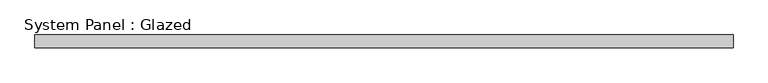
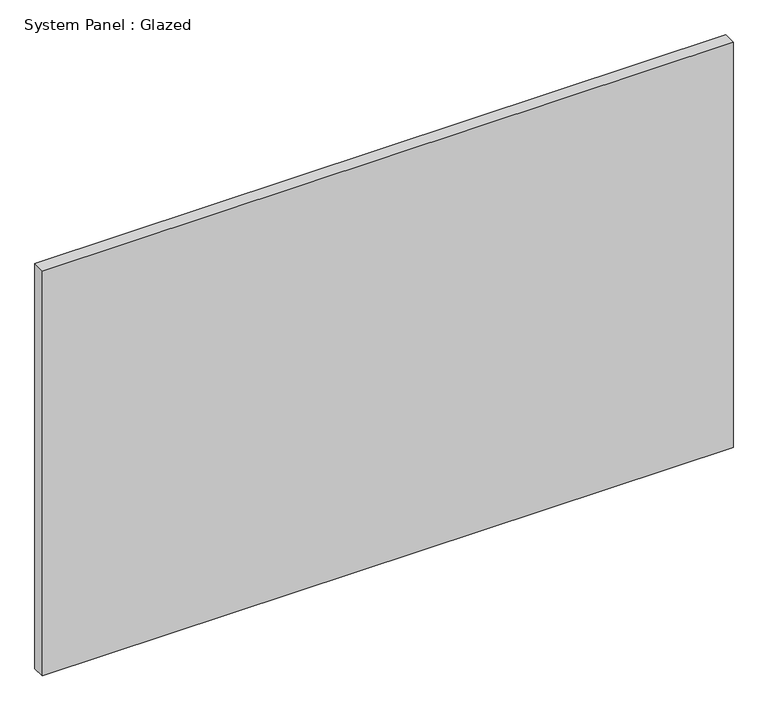
"""IFC4 building model written with IfcOpenShell, lengths in millimetres: plate geometry, System Panel : Glazed."""

from ifc_helpers import new_model, si_unit, origin, origin_with_axes, place, context, project, spatial, polyline, outline, extrude, source, transform, mapped, element, save


def system_panel_glazed_cad8d6ff(model_context):
    return source(origin(), model_context, "Body", "SweptSolid", [
        extrude(outline(polyline([(685.8000001, -44.45), (-685.8000001, -44.45), (-685.8000001, -19.05), (685.8000001, -19.05), (685.8000001, -44.45)])), origin_with_axes(), (0.0, 0.0, 1.0), 850.9),
    ])


if __name__ == "__main__":
    model = new_model("IFC4")
    model_context = context("Model", 3, world=origin())
    ifc_project = project(units=[si_unit("LENGTHUNIT", "METRE", prefix="MILLI")], contexts=[model_context])
    site = spatial("IfcSite", under=ifc_project)
    building = spatial("IfcBuilding", under=site)
    placement = place(None, origin())
    system_panel_glazed_shape = system_panel_glazed_cad8d6ff(model_context)
    element("IfcPlate", 1, ObjectType="System Panel : Glazed", at=placement, inside=building, context=model_context, shape_type="MappedRepresentation", body=[
        mapped(system_panel_glazed_shape, transform((0.0, 0.0, 0.0), x_axis=(1.0, 0.0, 0.0), y_axis=(0.0, 1.0, 0.0), z_axis=(0.0, 0.0, 1.0))),
    ])
    save(model, "model.ifc")

# Revit data of these elements
# Type "System Panel : Glazed"
#   Construction Type Id = "GSP4R"
#   Analytic Construction = "1/8 in Pilkington single glazing"
#   Visual Light Transmittance = 0.9
#   Solar Heat Gain Coefficient = 0.86
#   Heat Transfer Coefficient (U) = 1.18115 BTU/(h·ft²·°F)
#   Define Thermal Properties by = 1
# Element 1 (IfcPlate, "System Panel : Glazed")
#   Materials on its faces: "Glass"
# Materials
#   "Glass": class "Glass", colour RGB 0 128 192, transparency 0.75, Description = "Soda Lime Glass", Cost = 0
